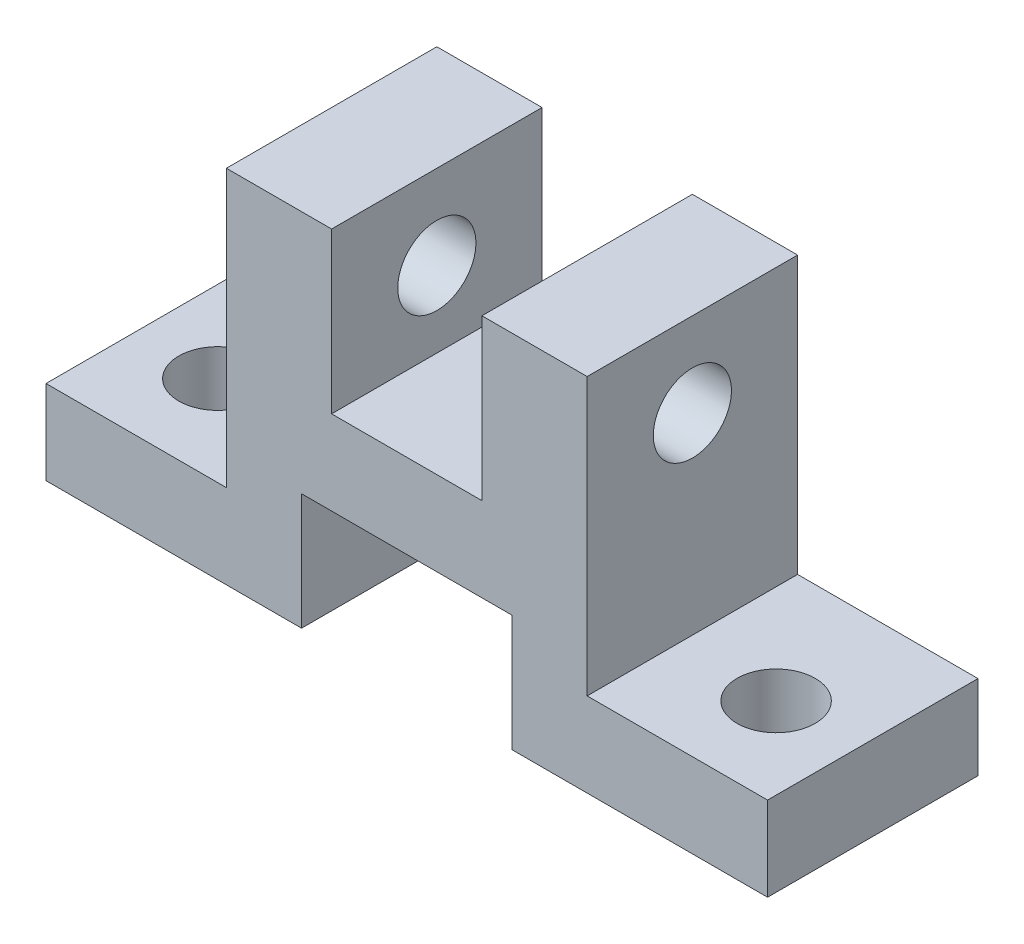
ISO-10303-21;
HEADER;
FILE_DESCRIPTION(('STEP AP214'),'2;1');
FILE_NAME('part.step','',(''),(''),'','','');
FILE_SCHEMA(('AUTOMOTIVE_DESIGN { 1 0 10303 214 1 1 1 1 }'));
ENDSEC;
DATA;
#1=APPLICATION_CONTEXT('core data for automotive mechanical design processes');
#2=APPLICATION_PROTOCOL_DEFINITION('international standard','automotive_design',2000,#1);
#3=PRODUCT_CONTEXT('',#1,'mechanical');
#4=PRODUCT('Part','Part','',(#3));
#5=PRODUCT_RELATED_PRODUCT_CATEGORY('part','',(#4));
#6=PRODUCT_DEFINITION_FORMATION('','',#4);
#7=PRODUCT_DEFINITION_CONTEXT('part definition',#1,'design');
#8=PRODUCT_DEFINITION('design','',#6,#7);
#9=PRODUCT_DEFINITION_SHAPE('','',#8);
#10=(LENGTH_UNIT() NAMED_UNIT(*) SI_UNIT(.MILLI.,.METRE.));
#11=(NAMED_UNIT(*) PLANE_ANGLE_UNIT() SI_UNIT($,.RADIAN.));
#12=(NAMED_UNIT(*) SI_UNIT($,.STERADIAN.) SOLID_ANGLE_UNIT());
#13=UNCERTAINTY_MEASURE_WITH_UNIT(LENGTH_MEASURE(1.E-05),#10,'distance_accuracy_value','');
#14=(GEOMETRIC_REPRESENTATION_CONTEXT(3) GLOBAL_UNCERTAINTY_ASSIGNED_CONTEXT((#13)) GLOBAL_UNIT_ASSIGNED_CONTEXT((#10,
#11,#12)) REPRESENTATION_CONTEXT('',''));
#15=CARTESIAN_POINT('',(0.,0.,0.));
#16=DIRECTION('',(0.,0.,1.));
#17=DIRECTION('',(1.,0.,0.));
#18=AXIS2_PLACEMENT_3D('',#15,#16,#17);
#19=CARTESIAN_POINT('',(0.,0.,35.));
#20=DIRECTION('',(0.,1.,0.));
#21=DIRECTION('',(0.,0.,1.));
#22=AXIS2_PLACEMENT_3D('',#19,#20,#21);
#23=PLANE('',#22);
#24=DIRECTION('',(1.,0.,0.));
#25=VECTOR('',#24,1.);
#26=CARTESIAN_POINT('',(0.,0.,0.));
#27=LINE('',#26,#25);
#28=CARTESIAN_POINT('',(-17.5,0.,0.));
#29=VERTEX_POINT('',#28);
#30=CARTESIAN_POINT('',(17.5,0.,0.));
#31=VERTEX_POINT('',#30);
#32=EDGE_CURVE('E120',#29,#31,#27,.T.);
#33=ORIENTED_EDGE('',*,*,#32,.T.);
#34=DIRECTION('',(0.,0.,-1.));
#35=VECTOR('',#34,1.);
#36=CARTESIAN_POINT('',(17.5,0.,35.));
#37=LINE('',#36,#35);
#38=CARTESIAN_POINT('',(17.5,0.,35.));
#39=VERTEX_POINT('',#38);
#40=EDGE_CURVE('E11',#39,#31,#37,.T.);
#41=ORIENTED_EDGE('',*,*,#40,.F.);
#42=DIRECTION('',(1.,0.,0.));
#43=VECTOR('',#42,1.);
#44=CARTESIAN_POINT('',(0.,0.,35.));
#45=LINE('',#44,#43);
#46=CARTESIAN_POINT('',(-17.5,0.,35.));
#47=VERTEX_POINT('',#46);
#48=EDGE_CURVE('E124',#47,#39,#45,.T.);
#49=ORIENTED_EDGE('',*,*,#48,.F.);
#50=DIRECTION('',(0.,0.,-1.));
#51=VECTOR('',#50,1.);
#52=CARTESIAN_POINT('',(-17.5,0.,35.));
#53=LINE('',#52,#51);
#54=EDGE_CURVE('E182',#47,#29,#53,.T.);
#55=ORIENTED_EDGE('',*,*,#54,.T.);
#56=EDGE_LOOP('',(#33,#41,#49,#55));
#57=FACE_BOUND('',#56,.T.);
#58=ADVANCED_FACE('F41',(#57),#23,.F.);
#59=CARTESIAN_POINT('',(17.5,0.,35.));
#60=DIRECTION('',(1.,0.,0.));
#61=DIRECTION('',(0.,1.,0.));
#62=AXIS2_PLACEMENT_3D('',#59,#60,#61);
#63=PLANE('',#62);
#64=DIRECTION('',(0.,-1.,0.));
#65=VECTOR('',#64,1.);
#66=CARTESIAN_POINT('',(17.5,0.,0.));
#67=LINE('',#66,#65);
#68=CARTESIAN_POINT('',(17.5,-19.3746378464225,0.));
#69=VERTEX_POINT('',#68);
#70=EDGE_CURVE('E188',#31,#69,#67,.T.);
#71=ORIENTED_EDGE('',*,*,#70,.T.);
#72=DIRECTION('',(0.,0.,-1.));
#73=VECTOR('',#72,1.);
#74=CARTESIAN_POINT('',(17.5,-19.3746378464225,35.));
#75=LINE('',#74,#73);
#76=CARTESIAN_POINT('',(17.5,-19.3746378464225,35.));
#77=VERTEX_POINT('',#76);
#78=EDGE_CURVE('E47',#77,#69,#75,.T.);
#79=ORIENTED_EDGE('',*,*,#78,.F.);
#80=DIRECTION('',(0.,-1.,0.));
#81=VECTOR('',#80,1.);
#82=CARTESIAN_POINT('',(17.5,0.,35.));
#83=LINE('',#82,#81);
#84=EDGE_CURVE('E304',#39,#77,#83,.T.);
#85=ORIENTED_EDGE('',*,*,#84,.F.);
#86=ORIENTED_EDGE('',*,*,#40,.T.);
#87=EDGE_LOOP('',(#71,#79,#85,#86));
#88=FACE_BOUND('',#87,.T.);
#89=ADVANCED_FACE('F306',(#88),#63,.F.);
#90=CARTESIAN_POINT('',(17.5,-19.3746378464225,35.));
#91=DIRECTION('',(0.,1.,0.));
#92=DIRECTION('',(-1.,0.,0.));
#93=AXIS2_PLACEMENT_3D('',#90,#91,#92);
#94=PLANE('',#93);
#95=CARTESIAN_POINT('',(46.4238989326504,-19.3746378464225,20.));
#96=DIRECTION('',(0.,1.,0.));
#97=DIRECTION('',(-1.,0.,0.));
#98=AXIS2_PLACEMENT_3D('',#95,#96,#97);
#99=CIRCLE('',#98,6.5);
#100=CARTESIAN_POINT('',(39.9238989326504,-19.3746378464225,20.));
#101=VERTEX_POINT('',#100);
#102=EDGE_CURVE('E379',#101,#101,#99,.T.);
#103=ORIENTED_EDGE('',*,*,#102,.T.);
#104=EDGE_LOOP('',(#103));
#105=FACE_BOUND('',#104,.T.);
#106=DIRECTION('',(1.,0.,0.));
#107=VECTOR('',#106,1.);
#108=CARTESIAN_POINT('',(17.5,-19.3746378464225,0.));
#109=LINE('',#108,#107);
#110=CARTESIAN_POINT('',(60.,-19.3746378464225,0.));
#111=VERTEX_POINT('',#110);
#112=EDGE_CURVE('E189',#69,#111,#109,.T.);
#113=ORIENTED_EDGE('',*,*,#112,.T.);
#114=DIRECTION('',(0.,0.,-1.));
#115=VECTOR('',#114,1.);
#116=CARTESIAN_POINT('',(60.,-19.3746378464225,35.));
#117=LINE('',#116,#115);
#118=CARTESIAN_POINT('',(60.,-19.3746378464225,35.));
#119=VERTEX_POINT('',#118);
#120=EDGE_CURVE('E247',#119,#111,#117,.T.);
#121=ORIENTED_EDGE('',*,*,#120,.F.);
#122=DIRECTION('',(1.,0.,0.));
#123=VECTOR('',#122,1.);
#124=CARTESIAN_POINT('',(17.5,-19.3746378464225,35.));
#125=LINE('',#124,#123);
#126=EDGE_CURVE('E254',#77,#119,#125,.T.);
#127=ORIENTED_EDGE('',*,*,#126,.F.);
#128=ORIENTED_EDGE('',*,*,#78,.T.);
#129=EDGE_LOOP('',(#113,#121,#127,#128));
#130=FACE_BOUND('',#129,.T.);
#131=ADVANCED_FACE('F251',(#105,#130),#94,.F.);
#132=CARTESIAN_POINT('',(60.,-19.3746378464225,35.));
#133=DIRECTION('',(-1.,0.,0.));
#134=DIRECTION('',(0.,0.,1.));
#135=AXIS2_PLACEMENT_3D('',#132,#133,#134);
#136=PLANE('',#135);
#137=DIRECTION('',(0.,1.,0.));
#138=VECTOR('',#137,1.);
#139=CARTESIAN_POINT('',(60.,-19.3746378464225,0.));
#140=LINE('',#139,#138);
#141=CARTESIAN_POINT('',(60.,-5.37463784642245,0.));
#142=VERTEX_POINT('',#141);
#143=EDGE_CURVE('E192',#111,#142,#140,.T.);
#144=ORIENTED_EDGE('',*,*,#143,.T.);
#145=DIRECTION('',(0.,0.,-1.));
#146=VECTOR('',#145,1.);
#147=CARTESIAN_POINT('',(60.,-5.37463784642245,35.));
#148=LINE('',#147,#146);
#149=CARTESIAN_POINT('',(60.,-5.37463784642245,35.));
#150=VERTEX_POINT('',#149);
#151=EDGE_CURVE('E241',#150,#142,#148,.T.);
#152=ORIENTED_EDGE('',*,*,#151,.F.);
#153=DIRECTION('',(0.,1.,0.));
#154=VECTOR('',#153,1.);
#155=CARTESIAN_POINT('',(60.,-19.3746378464225,35.));
#156=LINE('',#155,#154);
#157=EDGE_CURVE('E272',#119,#150,#156,.T.);
#158=ORIENTED_EDGE('',*,*,#157,.F.);
#159=ORIENTED_EDGE('',*,*,#120,.T.);
#160=EDGE_LOOP('',(#144,#152,#158,#159));
#161=FACE_BOUND('',#160,.T.);
#162=ADVANCED_FACE('F262',(#161),#136,.F.);
#163=CARTESIAN_POINT('',(60.,-5.37463784642245,35.));
#164=DIRECTION('',(0.,-1.,0.));
#165=DIRECTION('',(1.,0.,0.));
#166=AXIS2_PLACEMENT_3D('',#163,#164,#165);
#167=PLANE('',#166);
#168=CARTESIAN_POINT('',(46.4238989326504,-5.37463784642245,20.));
#169=DIRECTION('',(0.,1.,0.));
#170=DIRECTION('',(-1.,0.,0.));
#171=AXIS2_PLACEMENT_3D('',#168,#169,#170);
#172=CIRCLE('',#171,6.5);
#173=CARTESIAN_POINT('',(39.9238989326504,-5.37463784642246,20.));
#174=VERTEX_POINT('',#173);
#175=EDGE_CURVE('E382',#174,#174,#172,.T.);
#176=ORIENTED_EDGE('',*,*,#175,.F.);
#177=EDGE_LOOP('',(#176));
#178=FACE_BOUND('',#177,.T.);
#179=DIRECTION('',(-1.,0.,0.));
#180=VECTOR('',#179,1.);
#181=CARTESIAN_POINT('',(60.,-5.37463784642245,0.));
#182=LINE('',#181,#180);
#183=CARTESIAN_POINT('',(30.,-5.37463784642246,0.));
#184=VERTEX_POINT('',#183);
#185=EDGE_CURVE('E194',#142,#184,#182,.T.);
#186=ORIENTED_EDGE('',*,*,#185,.T.);
#187=DIRECTION('',(0.,0.,-1.));
#188=VECTOR('',#187,1.);
#189=CARTESIAN_POINT('',(30.,-5.37463784642246,35.));
#190=LINE('',#189,#188);
#191=CARTESIAN_POINT('',(30.,-5.37463784642246,35.));
#192=VERTEX_POINT('',#191);
#193=EDGE_CURVE('E238',#192,#184,#190,.T.);
#194=ORIENTED_EDGE('',*,*,#193,.F.);
#195=DIRECTION('',(-1.,0.,0.));
#196=VECTOR('',#195,1.);
#197=CARTESIAN_POINT('',(60.,-5.37463784642245,35.));
#198=LINE('',#197,#196);
#199=EDGE_CURVE('E269',#150,#192,#198,.T.);
#200=ORIENTED_EDGE('',*,*,#199,.F.);
#201=ORIENTED_EDGE('',*,*,#151,.T.);
#202=EDGE_LOOP('',(#186,#194,#200,#201));
#203=FACE_BOUND('',#202,.T.);
#204=ADVANCED_FACE('F268',(#178,#203),#167,.F.);
#205=CARTESIAN_POINT('',(30.,-5.37463784642246,35.));
#206=DIRECTION('',(-1.,0.,0.));
#207=DIRECTION('',(0.,0.,1.));
#208=AXIS2_PLACEMENT_3D('',#205,#206,#207);
#209=PLANE('',#208);
#210=CARTESIAN_POINT('',(30.,26.6253621535775,17.5));
#211=DIRECTION('',(-1.,0.,0.));
#212=DIRECTION('',(0.,0.,1.));
#213=AXIS2_PLACEMENT_3D('',#210,#211,#212);
#214=CIRCLE('',#213,6.5);
#215=CARTESIAN_POINT('',(30.,26.6253621535775,24.));
#216=VERTEX_POINT('',#215);
#217=EDGE_CURVE('E190',#216,#216,#214,.T.);
#218=ORIENTED_EDGE('',*,*,#217,.T.);
#219=EDGE_LOOP('',(#218));
#220=FACE_BOUND('',#219,.T.);
#221=DIRECTION('',(0.,1.,0.));
#222=VECTOR('',#221,1.);
#223=CARTESIAN_POINT('',(30.,-5.37463784642246,0.));
#224=LINE('',#223,#222);
#225=CARTESIAN_POINT('',(30.,40.6253621535775,0.));
#226=VERTEX_POINT('',#225);
#227=EDGE_CURVE('E193',#184,#226,#224,.T.);
#228=ORIENTED_EDGE('',*,*,#227,.T.);
#229=DIRECTION('',(0.,0.,-1.));
#230=VECTOR('',#229,1.);
#231=CARTESIAN_POINT('',(30.,40.6253621535775,35.));
#232=LINE('',#231,#230);
#233=CARTESIAN_POINT('',(30.,40.6253621535775,35.));
#234=VERTEX_POINT('',#233);
#235=EDGE_CURVE('E240',#234,#226,#232,.T.);
#236=ORIENTED_EDGE('',*,*,#235,.F.);
#237=DIRECTION('',(0.,1.,0.));
#238=VECTOR('',#237,1.);
#239=CARTESIAN_POINT('',(30.,-5.37463784642246,35.));
#240=LINE('',#239,#238);
#241=EDGE_CURVE('E275',#192,#234,#240,.T.);
#242=ORIENTED_EDGE('',*,*,#241,.F.);
#243=ORIENTED_EDGE('',*,*,#193,.T.);
#244=EDGE_LOOP('',(#228,#236,#242,#243));
#245=FACE_BOUND('',#244,.T.);
#246=ADVANCED_FACE('F321',(#220,#245),#209,.F.);
#247=CARTESIAN_POINT('',(30.,40.6253621535775,35.));
#248=DIRECTION('',(0.,-1.,0.));
#249=DIRECTION('',(0.,0.,-1.));
#250=AXIS2_PLACEMENT_3D('',#247,#248,#249);
#251=PLANE('',#250);
#252=DIRECTION('',(-1.,0.,0.));
#253=VECTOR('',#252,1.);
#254=CARTESIAN_POINT('',(30.,40.6253621535775,0.));
#255=LINE('',#254,#253);
#256=CARTESIAN_POINT('',(12.5,40.6253621535775,0.));
#257=VERTEX_POINT('',#256);
#258=EDGE_CURVE('E197',#226,#257,#255,.T.);
#259=ORIENTED_EDGE('',*,*,#258,.T.);
#260=DIRECTION('',(0.,0.,-1.));
#261=VECTOR('',#260,1.);
#262=CARTESIAN_POINT('',(12.5,40.6253621535775,35.));
#263=LINE('',#262,#261);
#264=CARTESIAN_POINT('',(12.5,40.6253621535775,35.));
#265=VERTEX_POINT('',#264);
#266=EDGE_CURVE('E231',#265,#257,#263,.T.);
#267=ORIENTED_EDGE('',*,*,#266,.F.);
#268=DIRECTION('',(-1.,0.,0.));
#269=VECTOR('',#268,1.);
#270=CARTESIAN_POINT('',(30.,40.6253621535775,35.));
#271=LINE('',#270,#269);
#272=EDGE_CURVE('E274',#234,#265,#271,.T.);
#273=ORIENTED_EDGE('',*,*,#272,.F.);
#274=ORIENTED_EDGE('',*,*,#235,.T.);
#275=EDGE_LOOP('',(#259,#267,#273,#274));
#276=FACE_BOUND('',#275,.T.);
#277=ADVANCED_FACE('F324',(#276),#251,.F.);
#278=CARTESIAN_POINT('',(12.5,40.6253621535775,35.));
#279=DIRECTION('',(1.,0.,0.));
#280=DIRECTION('',(0.,1.,0.));
#281=AXIS2_PLACEMENT_3D('',#278,#279,#280);
#282=PLANE('',#281);
#283=CARTESIAN_POINT('',(12.5,26.6253621535775,17.5));
#284=DIRECTION('',(1.,0.,0.));
#285=DIRECTION('',(0.,1.,0.));
#286=AXIS2_PLACEMENT_3D('',#283,#284,#285);
#287=CIRCLE('',#286,6.5);
#288=CARTESIAN_POINT('',(12.5,26.6253621535775,24.));
#289=VERTEX_POINT('',#288);
#290=EDGE_CURVE('E399',#289,#289,#287,.T.);
#291=ORIENTED_EDGE('',*,*,#290,.T.);
#292=EDGE_LOOP('',(#291));
#293=FACE_BOUND('',#292,.T.);
#294=DIRECTION('',(0.,-1.,0.));
#295=VECTOR('',#294,1.);
#296=CARTESIAN_POINT('',(12.5,40.6253621535775,0.));
#297=LINE('',#296,#295);
#298=CARTESIAN_POINT('',(12.5,14.,0.));
#299=VERTEX_POINT('',#298);
#300=EDGE_CURVE('E200',#257,#299,#297,.T.);
#301=ORIENTED_EDGE('',*,*,#300,.T.);
#302=DIRECTION('',(0.,0.,-1.));
#303=VECTOR('',#302,1.);
#304=CARTESIAN_POINT('',(12.5,14.,35.));
#305=LINE('',#304,#303);
#306=CARTESIAN_POINT('',(12.5,14.,35.));
#307=VERTEX_POINT('',#306);
#308=EDGE_CURVE('E232',#307,#299,#305,.T.);
#309=ORIENTED_EDGE('',*,*,#308,.F.);
#310=DIRECTION('',(0.,-1.,0.));
#311=VECTOR('',#310,1.);
#312=CARTESIAN_POINT('',(12.5,40.6253621535775,35.));
#313=LINE('',#312,#311);
#314=EDGE_CURVE('E283',#265,#307,#313,.T.);
#315=ORIENTED_EDGE('',*,*,#314,.F.);
#316=ORIENTED_EDGE('',*,*,#266,.T.);
#317=EDGE_LOOP('',(#301,#309,#315,#316));
#318=FACE_BOUND('',#317,.T.);
#319=ADVANCED_FACE('F328',(#293,#318),#282,.F.);
#320=CARTESIAN_POINT('',(12.5,14.,35.));
#321=DIRECTION('',(0.,-1.,0.));
#322=DIRECTION('',(0.,0.,-1.));
#323=AXIS2_PLACEMENT_3D('',#320,#321,#322);
#324=PLANE('',#323);
#325=DIRECTION('',(-1.,0.,0.));
#326=VECTOR('',#325,1.);
#327=CARTESIAN_POINT('',(12.5,14.,0.));
#328=LINE('',#327,#326);
#329=CARTESIAN_POINT('',(-12.5,14.,0.));
#330=VERTEX_POINT('',#329);
#331=EDGE_CURVE('E203',#299,#330,#328,.T.);
#332=ORIENTED_EDGE('',*,*,#331,.T.);
#333=DIRECTION('',(0.,0.,-1.));
#334=VECTOR('',#333,1.);
#335=CARTESIAN_POINT('',(-12.5,14.,35.));
#336=LINE('',#335,#334);
#337=CARTESIAN_POINT('',(-12.5,14.,35.));
#338=VERTEX_POINT('',#337);
#339=EDGE_CURVE('E226',#338,#330,#336,.T.);
#340=ORIENTED_EDGE('',*,*,#339,.F.);
#341=DIRECTION('',(-1.,0.,0.));
#342=VECTOR('',#341,1.);
#343=CARTESIAN_POINT('',(12.5,14.,35.));
#344=LINE('',#343,#342);
#345=EDGE_CURVE('E281',#307,#338,#344,.T.);
#346=ORIENTED_EDGE('',*,*,#345,.F.);
#347=ORIENTED_EDGE('',*,*,#308,.T.);
#348=EDGE_LOOP('',(#332,#340,#346,#347));
#349=FACE_BOUND('',#348,.T.);
#350=ADVANCED_FACE('F334',(#349),#324,.F.);
#351=CARTESIAN_POINT('',(-12.5,40.6253621535775,35.));
#352=DIRECTION('',(-1.,0.,0.));
#353=DIRECTION('',(0.,-1.,0.));
#354=AXIS2_PLACEMENT_3D('',#351,#352,#353);
#355=PLANE('',#354);
#356=CARTESIAN_POINT('',(-12.5,26.6253621535775,17.5));
#357=DIRECTION('',(-1.,0.,0.));
#358=DIRECTION('',(0.,-1.,0.));
#359=AXIS2_PLACEMENT_3D('',#356,#357,#358);
#360=CIRCLE('',#359,6.5);
#361=CARTESIAN_POINT('',(-12.5,26.6253621535775,24.));
#362=VERTEX_POINT('',#361);
#363=EDGE_CURVE('E397',#362,#362,#360,.T.);
#364=ORIENTED_EDGE('',*,*,#363,.T.);
#365=EDGE_LOOP('',(#364));
#366=FACE_BOUND('',#365,.T.);
#367=DIRECTION('',(0.,1.,0.));
#368=VECTOR('',#367,1.);
#369=CARTESIAN_POINT('',(-12.5,40.6253621535775,0.));
#370=LINE('',#369,#368);
#371=CARTESIAN_POINT('',(-12.5,40.6253621535775,0.));
#372=VERTEX_POINT('',#371);
#373=EDGE_CURVE('E201',#330,#372,#370,.T.);
#374=ORIENTED_EDGE('',*,*,#373,.T.);
#375=DIRECTION('',(0.,0.,-1.));
#376=VECTOR('',#375,1.);
#377=CARTESIAN_POINT('',(-12.5,40.6253621535775,35.));
#378=LINE('',#377,#376);
#379=CARTESIAN_POINT('',(-12.5,40.6253621535775,35.));
#380=VERTEX_POINT('',#379);
#381=EDGE_CURVE('E223',#380,#372,#378,.T.);
#382=ORIENTED_EDGE('',*,*,#381,.F.);
#383=DIRECTION('',(0.,1.,0.));
#384=VECTOR('',#383,1.);
#385=CARTESIAN_POINT('',(-12.5,40.6253621535775,35.));
#386=LINE('',#385,#384);
#387=EDGE_CURVE('E282',#338,#380,#386,.T.);
#388=ORIENTED_EDGE('',*,*,#387,.F.);
#389=ORIENTED_EDGE('',*,*,#339,.T.);
#390=EDGE_LOOP('',(#374,#382,#388,#389));
#391=FACE_BOUND('',#390,.T.);
#392=ADVANCED_FACE('F340',(#366,#391),#355,.F.);
#393=CARTESIAN_POINT('',(-30.,40.6253621535775,35.));
#394=DIRECTION('',(0.,-1.,0.));
#395=DIRECTION('',(0.,0.,-1.));
#396=AXIS2_PLACEMENT_3D('',#393,#394,#395);
#397=PLANE('',#396);
#398=DIRECTION('',(-1.,0.,0.));
#399=VECTOR('',#398,1.);
#400=CARTESIAN_POINT('',(-30.,40.6253621535775,0.));
#401=LINE('',#400,#399);
#402=CARTESIAN_POINT('',(-30.,40.6253621535775,0.));
#403=VERTEX_POINT('',#402);
#404=EDGE_CURVE('E202',#372,#403,#401,.T.);
#405=ORIENTED_EDGE('',*,*,#404,.T.);
#406=DIRECTION('',(0.,0.,-1.));
#407=VECTOR('',#406,1.);
#408=CARTESIAN_POINT('',(-30.,40.6253621535775,35.));
#409=LINE('',#408,#407);
#410=CARTESIAN_POINT('',(-30.,40.6253621535775,35.));
#411=VERTEX_POINT('',#410);
#412=EDGE_CURVE('E225',#411,#403,#409,.T.);
#413=ORIENTED_EDGE('',*,*,#412,.F.);
#414=DIRECTION('',(-1.,0.,0.));
#415=VECTOR('',#414,1.);
#416=CARTESIAN_POINT('',(-30.,40.6253621535775,35.));
#417=LINE('',#416,#415);
#418=EDGE_CURVE('E290',#380,#411,#417,.T.);
#419=ORIENTED_EDGE('',*,*,#418,.F.);
#420=ORIENTED_EDGE('',*,*,#381,.T.);
#421=EDGE_LOOP('',(#405,#413,#419,#420));
#422=FACE_BOUND('',#421,.T.);
#423=ADVANCED_FACE('F342',(#422),#397,.F.);
#424=CARTESIAN_POINT('',(-30.,-5.37463784642246,35.));
#425=DIRECTION('',(1.,0.,0.));
#426=DIRECTION('',(0.,0.,-1.));
#427=AXIS2_PLACEMENT_3D('',#424,#425,#426);
#428=PLANE('',#427);
#429=CARTESIAN_POINT('',(-30.,26.6253621535775,17.5));
#430=DIRECTION('',(-1.,0.,0.));
#431=DIRECTION('',(0.,0.,1.));
#432=AXIS2_PLACEMENT_3D('',#429,#430,#431);
#433=CIRCLE('',#432,6.5);
#434=CARTESIAN_POINT('',(-30.,26.6253621535775,24.));
#435=VERTEX_POINT('',#434);
#436=EDGE_CURVE('E387',#435,#435,#433,.T.);
#437=ORIENTED_EDGE('',*,*,#436,.F.);
#438=EDGE_LOOP('',(#437));
#439=FACE_BOUND('',#438,.T.);
#440=DIRECTION('',(0.,-1.,0.));
#441=VECTOR('',#440,1.);
#442=CARTESIAN_POINT('',(-30.,-5.37463784642246,0.));
#443=LINE('',#442,#441);
#444=CARTESIAN_POINT('',(-30.,-5.37463784642246,0.));
#445=VERTEX_POINT('',#444);
#446=EDGE_CURVE('E210',#403,#445,#443,.T.);
#447=ORIENTED_EDGE('',*,*,#446,.T.);
#448=DIRECTION('',(0.,0.,-1.));
#449=VECTOR('',#448,1.);
#450=CARTESIAN_POINT('',(-30.,-5.37463784642246,35.));
#451=LINE('',#450,#449);
#452=CARTESIAN_POINT('',(-30.,-5.37463784642246,35.));
#453=VERTEX_POINT('',#452);
#454=EDGE_CURVE('E218',#453,#445,#451,.T.);
#455=ORIENTED_EDGE('',*,*,#454,.F.);
#456=DIRECTION('',(0.,-1.,0.));
#457=VECTOR('',#456,1.);
#458=CARTESIAN_POINT('',(-30.,-5.37463784642246,35.));
#459=LINE('',#458,#457);
#460=EDGE_CURVE('E286',#411,#453,#459,.T.);
#461=ORIENTED_EDGE('',*,*,#460,.F.);
#462=ORIENTED_EDGE('',*,*,#412,.T.);
#463=EDGE_LOOP('',(#447,#455,#461,#462));
#464=FACE_BOUND('',#463,.T.);
#465=ADVANCED_FACE('F293',(#439,#464),#428,.F.);
#466=CARTESIAN_POINT('',(-60.,-5.37463784642245,35.));
#467=DIRECTION('',(0.,-1.,0.));
#468=DIRECTION('',(1.,0.,0.));
#469=AXIS2_PLACEMENT_3D('',#466,#467,#468);
#470=PLANE('',#469);
#471=CARTESIAN_POINT('',(-46.4238989326504,-5.37463784642247,20.));
#472=DIRECTION('',(0.,1.,0.));
#473=DIRECTION('',(1.,0.,0.));
#474=AXIS2_PLACEMENT_3D('',#471,#472,#473);
#475=CIRCLE('',#474,6.5);
#476=CARTESIAN_POINT('',(-39.9238989326504,-5.37463784642246,20.));
#477=VERTEX_POINT('',#476);
#478=EDGE_CURVE('E383',#477,#477,#475,.T.);
#479=ORIENTED_EDGE('',*,*,#478,.F.);
#480=EDGE_LOOP('',(#479));
#481=FACE_BOUND('',#480,.T.);
#482=DIRECTION('',(-1.,0.,0.));
#483=VECTOR('',#482,1.);
#484=CARTESIAN_POINT('',(-60.,-5.37463784642245,0.));
#485=LINE('',#484,#483);
#486=CARTESIAN_POINT('',(-60.,-5.37463784642245,0.));
#487=VERTEX_POINT('',#486);
#488=EDGE_CURVE('E207',#445,#487,#485,.T.);
#489=ORIENTED_EDGE('',*,*,#488,.T.);
#490=DIRECTION('',(0.,0.,-1.));
#491=VECTOR('',#490,1.);
#492=CARTESIAN_POINT('',(-60.,-5.37463784642245,35.));
#493=LINE('',#492,#491);
#494=CARTESIAN_POINT('',(-60.,-5.37463784642245,35.));
#495=VERTEX_POINT('',#494);
#496=EDGE_CURVE('E177',#495,#487,#493,.T.);
#497=ORIENTED_EDGE('',*,*,#496,.F.);
#498=DIRECTION('',(-1.,0.,0.));
#499=VECTOR('',#498,1.);
#500=CARTESIAN_POINT('',(-60.,-5.37463784642245,35.));
#501=LINE('',#500,#499);
#502=EDGE_CURVE('E170',#453,#495,#501,.T.);
#503=ORIENTED_EDGE('',*,*,#502,.F.);
#504=ORIENTED_EDGE('',*,*,#454,.T.);
#505=EDGE_LOOP('',(#489,#497,#503,#504));
#506=FACE_BOUND('',#505,.T.);
#507=ADVANCED_FACE('F299',(#481,#506),#470,.F.);
#508=CARTESIAN_POINT('',(-60.,-19.3746378464225,35.));
#509=DIRECTION('',(1.,0.,0.));
#510=DIRECTION('',(0.,0.,-1.));
#511=AXIS2_PLACEMENT_3D('',#508,#509,#510);
#512=PLANE('',#511);
#513=DIRECTION('',(0.,-1.,0.));
#514=VECTOR('',#513,1.);
#515=CARTESIAN_POINT('',(-60.,-19.3746378464225,0.));
#516=LINE('',#515,#514);
#517=CARTESIAN_POINT('',(-60.,-19.3746378464225,0.));
#518=VERTEX_POINT('',#517);
#519=EDGE_CURVE('E172',#487,#518,#516,.T.);
#520=ORIENTED_EDGE('',*,*,#519,.T.);
#521=DIRECTION('',(0.,0.,-1.));
#522=VECTOR('',#521,1.);
#523=CARTESIAN_POINT('',(-60.,-19.3746378464225,35.));
#524=LINE('',#523,#522);
#525=CARTESIAN_POINT('',(-60.,-19.3746378464225,35.));
#526=VERTEX_POINT('',#525);
#527=EDGE_CURVE('E175',#526,#518,#524,.T.);
#528=ORIENTED_EDGE('',*,*,#527,.F.);
#529=DIRECTION('',(0.,-1.,0.));
#530=VECTOR('',#529,1.);
#531=CARTESIAN_POINT('',(-60.,-19.3746378464225,35.));
#532=LINE('',#531,#530);
#533=EDGE_CURVE('E161',#495,#526,#532,.T.);
#534=ORIENTED_EDGE('',*,*,#533,.F.);
#535=ORIENTED_EDGE('',*,*,#496,.T.);
#536=EDGE_LOOP('',(#520,#528,#534,#535));
#537=FACE_BOUND('',#536,.T.);
#538=ADVANCED_FACE('F171',(#537),#512,.F.);
#539=CARTESIAN_POINT('',(-17.5,-19.3746378464225,35.));
#540=DIRECTION('',(0.,1.,0.));
#541=DIRECTION('',(-1.,0.,0.));
#542=AXIS2_PLACEMENT_3D('',#539,#540,#541);
#543=PLANE('',#542);
#544=CARTESIAN_POINT('',(-46.4238989326504,-19.3746378464225,20.));
#545=DIRECTION('',(0.,1.,0.));
#546=DIRECTION('',(1.,0.,0.));
#547=AXIS2_PLACEMENT_3D('',#544,#545,#546);
#548=CIRCLE('',#547,6.5);
#549=CARTESIAN_POINT('',(-39.9238989326504,-19.3746378464225,20.));
#550=VERTEX_POINT('',#549);
#551=EDGE_CURVE('E386',#550,#550,#548,.T.);
#552=ORIENTED_EDGE('',*,*,#551,.T.);
#553=EDGE_LOOP('',(#552));
#554=FACE_BOUND('',#553,.T.);
#555=DIRECTION('',(1.,0.,0.));
#556=VECTOR('',#555,1.);
#557=CARTESIAN_POINT('',(-17.5,-19.3746378464225,0.));
#558=LINE('',#557,#556);
#559=CARTESIAN_POINT('',(-17.5,-19.3746378464225,0.));
#560=VERTEX_POINT('',#559);
#561=EDGE_CURVE('E109',#518,#560,#558,.T.);
#562=ORIENTED_EDGE('',*,*,#561,.T.);
#563=DIRECTION('',(0.,0.,-1.));
#564=VECTOR('',#563,1.);
#565=CARTESIAN_POINT('',(-17.5,-19.3746378464225,35.));
#566=LINE('',#565,#564);
#567=CARTESIAN_POINT('',(-17.5,-19.3746378464225,35.));
#568=VERTEX_POINT('',#567);
#569=EDGE_CURVE('E180',#568,#560,#566,.T.);
#570=ORIENTED_EDGE('',*,*,#569,.F.);
#571=DIRECTION('',(1.,0.,0.));
#572=VECTOR('',#571,1.);
#573=CARTESIAN_POINT('',(-17.5,-19.3746378464225,35.));
#574=LINE('',#573,#572);
#575=EDGE_CURVE('E164',#526,#568,#574,.T.);
#576=ORIENTED_EDGE('',*,*,#575,.F.);
#577=ORIENTED_EDGE('',*,*,#527,.T.);
#578=EDGE_LOOP('',(#562,#570,#576,#577));
#579=FACE_BOUND('',#578,.T.);
#580=ADVANCED_FACE('F176',(#554,#579),#543,.F.);
#581=CARTESIAN_POINT('',(-17.5,0.,35.));
#582=DIRECTION('',(-1.,0.,0.));
#583=DIRECTION('',(0.,-1.,0.));
#584=AXIS2_PLACEMENT_3D('',#581,#582,#583);
#585=PLANE('',#584);
#586=DIRECTION('',(0.,1.,0.));
#587=VECTOR('',#586,1.);
#588=CARTESIAN_POINT('',(-17.5,0.,0.));
#589=LINE('',#588,#587);
#590=EDGE_CURVE('E213',#560,#29,#589,.T.);
#591=ORIENTED_EDGE('',*,*,#590,.T.);
#592=ORIENTED_EDGE('',*,*,#54,.F.);
#593=DIRECTION('',(0.,1.,0.));
#594=VECTOR('',#593,1.);
#595=CARTESIAN_POINT('',(-17.5,0.,35.));
#596=LINE('',#595,#594);
#597=EDGE_CURVE('E60',#568,#47,#596,.T.);
#598=ORIENTED_EDGE('',*,*,#597,.F.);
#599=ORIENTED_EDGE('',*,*,#569,.T.);
#600=EDGE_LOOP('',(#591,#592,#598,#599));
#601=FACE_BOUND('',#600,.T.);
#602=ADVANCED_FACE('F302',(#601),#585,.F.);
#603=CARTESIAN_POINT('',(0.,0.,35.));
#604=DIRECTION('',(0.,0.,1.));
#605=DIRECTION('',(1.,0.,0.));
#606=AXIS2_PLACEMENT_3D('',#603,#604,#605);
#607=PLANE('',#606);
#608=ORIENTED_EDGE('',*,*,#48,.T.);
#609=ORIENTED_EDGE('',*,*,#84,.T.);
#610=ORIENTED_EDGE('',*,*,#126,.T.);
#611=ORIENTED_EDGE('',*,*,#157,.T.);
#612=ORIENTED_EDGE('',*,*,#199,.T.);
#613=ORIENTED_EDGE('',*,*,#241,.T.);
#614=ORIENTED_EDGE('',*,*,#272,.T.);
#615=ORIENTED_EDGE('',*,*,#314,.T.);
#616=ORIENTED_EDGE('',*,*,#345,.T.);
#617=ORIENTED_EDGE('',*,*,#387,.T.);
#618=ORIENTED_EDGE('',*,*,#418,.T.);
#619=ORIENTED_EDGE('',*,*,#460,.T.);
#620=ORIENTED_EDGE('',*,*,#502,.T.);
#621=ORIENTED_EDGE('',*,*,#533,.T.);
#622=ORIENTED_EDGE('',*,*,#575,.T.);
#623=ORIENTED_EDGE('',*,*,#597,.T.);
#624=EDGE_LOOP('',(#608,#609,#610,#611,#612,#613,#614,#615,#616,#617,#618,#619,#620,#621,#622,#623));
#625=FACE_BOUND('',#624,.T.);
#626=ADVANCED_FACE('F162',(#625),#607,.T.);
#627=CARTESIAN_POINT('',(0.,0.,0.));
#628=DIRECTION('',(0.,0.,1.));
#629=DIRECTION('',(1.,0.,0.));
#630=AXIS2_PLACEMENT_3D('',#627,#628,#629);
#631=PLANE('',#630);
#632=ORIENTED_EDGE('',*,*,#32,.F.);
#633=ORIENTED_EDGE('',*,*,#590,.F.);
#634=ORIENTED_EDGE('',*,*,#561,.F.);
#635=ORIENTED_EDGE('',*,*,#519,.F.);
#636=ORIENTED_EDGE('',*,*,#488,.F.);
#637=ORIENTED_EDGE('',*,*,#446,.F.);
#638=ORIENTED_EDGE('',*,*,#404,.F.);
#639=ORIENTED_EDGE('',*,*,#373,.F.);
#640=ORIENTED_EDGE('',*,*,#331,.F.);
#641=ORIENTED_EDGE('',*,*,#300,.F.);
#642=ORIENTED_EDGE('',*,*,#258,.F.);
#643=ORIENTED_EDGE('',*,*,#227,.F.);
#644=ORIENTED_EDGE('',*,*,#185,.F.);
#645=ORIENTED_EDGE('',*,*,#143,.F.);
#646=ORIENTED_EDGE('',*,*,#112,.F.);
#647=ORIENTED_EDGE('',*,*,#70,.F.);
#648=EDGE_LOOP('',(#632,#633,#634,#635,#636,#637,#638,#639,#640,#641,#642,#643,#644,#645,#646,#647));
#649=FACE_BOUND('',#648,.T.);
#650=ADVANCED_FACE('F259',(#649),#631,.F.);
#651=CARTESIAN_POINT('',(60.,26.6253621535775,17.5));
#652=DIRECTION('',(-1.,0.,0.));
#653=DIRECTION('',(0.,0.,1.));
#654=AXIS2_PLACEMENT_3D('',#651,#652,#653);
#655=CYLINDRICAL_SURFACE('',#654,6.5);
#656=CARTESIAN_POINT('',(-30.,26.6253621535775,24.));
#657=CARTESIAN_POINT('',(-29.8177083333333,26.6253621535775,24.));
#658=CARTESIAN_POINT('',(-29.6354166666667,26.6253621535775,24.));
#659=CARTESIAN_POINT('',(-29.2708333333333,26.6253621535775,24.));
#660=CARTESIAN_POINT('',(-29.0885416666666,26.6253621535775,24.));
#661=CARTESIAN_POINT('',(-28.7239583333333,26.6253621535775,24.));
#662=CARTESIAN_POINT('',(-28.5416666666667,26.6253621535775,24.));
#663=CARTESIAN_POINT('',(-28.1770833333333,26.6253621535775,24.));
#664=CARTESIAN_POINT('',(-27.9947916666667,26.6253621535775,24.));
#665=CARTESIAN_POINT('',(-27.6302083333333,26.6253621535775,24.));
#666=CARTESIAN_POINT('',(-27.4479166666667,26.6253621535775,24.));
#667=CARTESIAN_POINT('',(-27.0833333333333,26.6253621535775,24.));
#668=CARTESIAN_POINT('',(-26.9010416666667,26.6253621535775,24.));
#669=CARTESIAN_POINT('',(-26.5364583333333,26.6253621535775,24.));
#670=CARTESIAN_POINT('',(-26.3541666666667,26.6253621535775,24.));
#671=CARTESIAN_POINT('',(-25.9895833333333,26.6253621535775,24.));
#672=CARTESIAN_POINT('',(-25.8072916666667,26.6253621535775,24.));
#673=CARTESIAN_POINT('',(-25.4427083333333,26.6253621535775,24.));
#674=CARTESIAN_POINT('',(-25.2604166666667,26.6253621535775,24.));
#675=CARTESIAN_POINT('',(-24.8958333333333,26.6253621535775,24.));
#676=CARTESIAN_POINT('',(-24.7135416666667,26.6253621535775,24.));
#677=CARTESIAN_POINT('',(-24.3489583333333,26.6253621535775,24.));
#678=CARTESIAN_POINT('',(-24.1666666666667,26.6253621535775,24.));
#679=CARTESIAN_POINT('',(-23.8020833333333,26.6253621535775,24.));
#680=CARTESIAN_POINT('',(-23.6197916666667,26.6253621535775,24.));
#681=CARTESIAN_POINT('',(-23.2552083333333,26.6253621535775,24.));
#682=CARTESIAN_POINT('',(-23.0729166666667,26.6253621535775,24.));
#683=CARTESIAN_POINT('',(-22.7083333333333,26.6253621535775,24.));
#684=CARTESIAN_POINT('',(-22.5260416666667,26.6253621535775,24.));
#685=CARTESIAN_POINT('',(-22.1614583333333,26.6253621535775,24.));
#686=CARTESIAN_POINT('',(-21.9791666666667,26.6253621535775,24.));
#687=CARTESIAN_POINT('',(-21.6145833333333,26.6253621535775,24.));
#688=CARTESIAN_POINT('',(-21.4322916666667,26.6253621535775,24.));
#689=CARTESIAN_POINT('',(-21.0677083333333,26.6253621535775,24.));
#690=CARTESIAN_POINT('',(-20.8854166666667,26.6253621535775,24.));
#691=CARTESIAN_POINT('',(-20.5208333333333,26.6253621535775,24.));
#692=CARTESIAN_POINT('',(-20.3385416666667,26.6253621535775,24.));
#693=CARTESIAN_POINT('',(-19.9739583333333,26.6253621535775,24.));
#694=CARTESIAN_POINT('',(-19.7916666666667,26.6253621535775,24.));
#695=CARTESIAN_POINT('',(-19.4270833333333,26.6253621535775,24.));
#696=CARTESIAN_POINT('',(-19.2447916666667,26.6253621535775,24.));
#697=CARTESIAN_POINT('',(-18.8802083333333,26.6253621535775,24.));
#698=CARTESIAN_POINT('',(-18.6979166666667,26.6253621535775,24.));
#699=CARTESIAN_POINT('',(-18.3333333333333,26.6253621535775,24.));
#700=CARTESIAN_POINT('',(-18.1510416666667,26.6253621535775,24.));
#701=CARTESIAN_POINT('',(-17.7864583333333,26.6253621535775,24.));
#702=CARTESIAN_POINT('',(-17.6041666666667,26.6253621535775,24.));
#703=CARTESIAN_POINT('',(-17.2395833333333,26.6253621535775,24.));
#704=CARTESIAN_POINT('',(-17.0572916666667,26.6253621535775,24.));
#705=CARTESIAN_POINT('',(-16.6927083333333,26.6253621535775,24.));
#706=CARTESIAN_POINT('',(-16.5104166666667,26.6253621535775,24.));
#707=CARTESIAN_POINT('',(-16.1458333333333,26.6253621535775,24.));
#708=CARTESIAN_POINT('',(-15.9635416666667,26.6253621535775,24.));
#709=CARTESIAN_POINT('',(-15.5989583333333,26.6253621535775,24.));
#710=CARTESIAN_POINT('',(-15.4166666666667,26.6253621535775,24.));
#711=CARTESIAN_POINT('',(-15.0520833333333,26.6253621535775,24.));
#712=CARTESIAN_POINT('',(-14.8697916666667,26.6253621535775,24.));
#713=CARTESIAN_POINT('',(-14.5052083333333,26.6253621535775,24.));
#714=CARTESIAN_POINT('',(-14.3229166666667,26.6253621535775,24.));
#715=CARTESIAN_POINT('',(-13.9583333333333,26.6253621535775,24.));
#716=CARTESIAN_POINT('',(-13.7760416666667,26.6253621535775,24.));
#717=CARTESIAN_POINT('',(-13.4114583333333,26.6253621535775,24.));
#718=CARTESIAN_POINT('',(-13.2291666666667,26.6253621535775,24.));
#719=CARTESIAN_POINT('',(-12.8645833333333,26.6253621535775,24.));
#720=CARTESIAN_POINT('',(-12.6822916666667,26.6253621535775,24.));
#721=CARTESIAN_POINT('',(-12.5,26.6253621535775,24.));
#722=B_SPLINE_CURVE_WITH_KNOTS('',3,(#656,#657,#658,#659,#660,#661,#662,#663,#664,#665,#666,
#667,#668,#669,#670,#671,#672,#673,#674,#675,#676,#677,#678,#679,#680,#681,#682,#683,#684,#685,
#686,#687,#688,#689,#690,#691,#692,#693,#694,#695,#696,#697,#698,#699,#700,#701,#702,#703,#704,
#705,#706,#707,#708,#709,#710,#711,#712,#713,#714,#715,#716,#717,#718,#719,#720,#721),
.UNSPECIFIED.,.F.,.F.,(4,2,2,2,2,2,2,2,2,2,2,2,2,2,2,2,2,2,2,2,2,2,2,2,2,2,2,2,2,2,2,2,4),(0.,
0.546875000000002,1.09375,1.64062499999999,2.1875,2.734375,3.28125,3.828125,4.37499999999999,
4.92187499999999,5.46874999999999,6.015625,6.5625,7.109375,7.65624999999999,8.20312499999999,
8.74999999999999,9.296875,9.84375,10.390625,10.9375,11.484375,12.03125,12.578125,13.125,
13.671875,14.21875,14.765625,15.3125,15.859375,16.40625,16.953125,17.5),.UNSPECIFIED.);
#723=EDGE_CURVE('BSEAM363',#435,#362,#722,.T.);
#724=ORIENTED_EDGE('',*,*,#436,.T.);
#725=ORIENTED_EDGE('',*,*,#363,.F.);
#726=ORIENTED_EDGE('',*,*,#723,.T.);
#727=ORIENTED_EDGE('',*,*,#723,.F.);
#728=EDGE_LOOP('',(#724,#726,#725,#727));
#729=FACE_BOUND('',#728,.T.);
#730=ADVANCED_FACE('F363',(#729),#655,.F.);
#731=CARTESIAN_POINT('',(12.5,26.6253621535775,24.));
#732=CARTESIAN_POINT('',(12.6822916666667,26.6253621535775,24.));
#733=CARTESIAN_POINT('',(12.8645833333333,26.6253621535775,24.));
#734=CARTESIAN_POINT('',(13.2291666666667,26.6253621535775,24.));
#735=CARTESIAN_POINT('',(13.4114583333333,26.6253621535775,24.));
#736=CARTESIAN_POINT('',(13.7760416666667,26.6253621535775,24.));
#737=CARTESIAN_POINT('',(13.9583333333333,26.6253621535775,24.));
#738=CARTESIAN_POINT('',(14.3229166666667,26.6253621535775,24.));
#739=CARTESIAN_POINT('',(14.5052083333333,26.6253621535775,24.));
#740=CARTESIAN_POINT('',(14.8697916666667,26.6253621535775,24.));
#741=CARTESIAN_POINT('',(15.0520833333333,26.6253621535775,24.));
#742=CARTESIAN_POINT('',(15.4166666666667,26.6253621535775,24.));
#743=CARTESIAN_POINT('',(15.5989583333333,26.6253621535775,24.));
#744=CARTESIAN_POINT('',(15.9635416666667,26.6253621535775,24.));
#745=CARTESIAN_POINT('',(16.1458333333333,26.6253621535775,24.));
#746=CARTESIAN_POINT('',(16.5104166666667,26.6253621535775,24.));
#747=CARTESIAN_POINT('',(16.6927083333333,26.6253621535775,24.));
#748=CARTESIAN_POINT('',(17.0572916666667,26.6253621535775,24.));
#749=CARTESIAN_POINT('',(17.2395833333333,26.6253621535775,24.));
#750=CARTESIAN_POINT('',(17.6041666666667,26.6253621535775,24.));
#751=CARTESIAN_POINT('',(17.7864583333333,26.6253621535775,24.));
#752=CARTESIAN_POINT('',(18.1510416666667,26.6253621535775,24.));
#753=CARTESIAN_POINT('',(18.3333333333333,26.6253621535775,24.));
#754=CARTESIAN_POINT('',(18.6979166666667,26.6253621535775,24.));
#755=CARTESIAN_POINT('',(18.8802083333333,26.6253621535775,24.));
#756=CARTESIAN_POINT('',(19.2447916666667,26.6253621535775,24.));
#757=CARTESIAN_POINT('',(19.4270833333333,26.6253621535775,24.));
#758=CARTESIAN_POINT('',(19.7916666666667,26.6253621535775,24.));
#759=CARTESIAN_POINT('',(19.9739583333333,26.6253621535775,24.));
#760=CARTESIAN_POINT('',(20.3385416666667,26.6253621535775,24.));
#761=CARTESIAN_POINT('',(20.5208333333333,26.6253621535775,24.));
#762=CARTESIAN_POINT('',(20.8854166666667,26.6253621535775,24.));
#763=CARTESIAN_POINT('',(21.0677083333333,26.6253621535775,24.));
#764=CARTESIAN_POINT('',(21.4322916666667,26.6253621535775,24.));
#765=CARTESIAN_POINT('',(21.6145833333333,26.6253621535775,24.));
#766=CARTESIAN_POINT('',(21.9791666666667,26.6253621535775,24.));
#767=CARTESIAN_POINT('',(22.1614583333333,26.6253621535775,24.));
#768=CARTESIAN_POINT('',(22.5260416666667,26.6253621535775,24.));
#769=CARTESIAN_POINT('',(22.7083333333333,26.6253621535775,24.));
#770=CARTESIAN_POINT('',(23.0729166666667,26.6253621535775,24.));
#771=CARTESIAN_POINT('',(23.2552083333333,26.6253621535775,24.));
#772=CARTESIAN_POINT('',(23.6197916666667,26.6253621535775,24.));
#773=CARTESIAN_POINT('',(23.8020833333333,26.6253621535775,24.));
#774=CARTESIAN_POINT('',(24.1666666666667,26.6253621535775,24.));
#775=CARTESIAN_POINT('',(24.3489583333333,26.6253621535775,24.));
#776=CARTESIAN_POINT('',(24.7135416666667,26.6253621535775,24.));
#777=CARTESIAN_POINT('',(24.8958333333333,26.6253621535775,24.));
#778=CARTESIAN_POINT('',(25.2604166666667,26.6253621535775,24.));
#779=CARTESIAN_POINT('',(25.4427083333333,26.6253621535775,24.));
#780=CARTESIAN_POINT('',(25.8072916666667,26.6253621535775,24.));
#781=CARTESIAN_POINT('',(25.9895833333333,26.6253621535775,24.));
#782=CARTESIAN_POINT('',(26.3541666666667,26.6253621535775,24.));
#783=CARTESIAN_POINT('',(26.5364583333333,26.6253621535775,24.));
#784=CARTESIAN_POINT('',(26.9010416666667,26.6253621535775,24.));
#785=CARTESIAN_POINT('',(27.0833333333333,26.6253621535775,24.));
#786=CARTESIAN_POINT('',(27.4479166666667,26.6253621535775,24.));
#787=CARTESIAN_POINT('',(27.6302083333333,26.6253621535775,24.));
#788=CARTESIAN_POINT('',(27.9947916666667,26.6253621535775,24.));
#789=CARTESIAN_POINT('',(28.1770833333333,26.6253621535775,24.));
#790=CARTESIAN_POINT('',(28.5416666666667,26.6253621535775,24.));
#791=CARTESIAN_POINT('',(28.7239583333333,26.6253621535775,24.));
#792=CARTESIAN_POINT('',(29.0885416666667,26.6253621535775,24.));
#793=CARTESIAN_POINT('',(29.2708333333333,26.6253621535775,24.));
#794=CARTESIAN_POINT('',(29.6354166666667,26.6253621535775,24.));
#795=CARTESIAN_POINT('',(29.8177083333333,26.6253621535775,24.));
#796=CARTESIAN_POINT('',(30.,26.6253621535775,24.));
#797=B_SPLINE_CURVE_WITH_KNOTS('',3,(#731,#732,#733,#734,#735,#736,#737,#738,#739,#740,#741,
#742,#743,#744,#745,#746,#747,#748,#749,#750,#751,#752,#753,#754,#755,#756,#757,#758,#759,#760,
#761,#762,#763,#764,#765,#766,#767,#768,#769,#770,#771,#772,#773,#774,#775,#776,#777,#778,#779,
#780,#781,#782,#783,#784,#785,#786,#787,#788,#789,#790,#791,#792,#793,#794,#795,#796),
.UNSPECIFIED.,.F.,.F.,(4,2,2,2,2,2,2,2,2,2,2,2,2,2,2,2,2,2,2,2,2,2,2,2,2,2,2,2,2,2,2,2,4),(0.,
0.546875000000002,1.09375,1.640625,2.1875,2.734375,3.28125,3.828125,4.375,4.92187500000001,
5.46875000000001,6.015625,6.56250000000001,7.10937500000001,7.65625,8.20312500000001,
8.75000000000001,9.29687500000001,9.84375000000001,10.390625,10.9375,11.484375,12.03125,
12.578125,13.125,13.671875,14.21875,14.765625,15.3125,15.859375,16.40625,16.953125,17.5),.UNSPECIFIED.);
#798=EDGE_CURVE('BSEAM365',#289,#216,#797,.T.);
#799=ORIENTED_EDGE('',*,*,#290,.F.);
#800=ORIENTED_EDGE('',*,*,#217,.F.);
#801=ORIENTED_EDGE('',*,*,#798,.T.);
#802=ORIENTED_EDGE('',*,*,#798,.F.);
#803=EDGE_LOOP('',(#799,#801,#800,#802));
#804=FACE_BOUND('',#803,.T.);
#805=ADVANCED_FACE('F365',(#804),#655,.F.);
#806=CARTESIAN_POINT('',(-46.4238989326504,-19.3746378464225,20.));
#807=DIRECTION('',(0.,1.,0.));
#808=DIRECTION('',(-1.,0.,0.));
#809=AXIS2_PLACEMENT_3D('',#806,#807,#808);
#810=CYLINDRICAL_SURFACE('',#809,6.5);
#811=ORIENTED_EDGE('',*,*,#551,.F.);
#812=EDGE_LOOP('',(#811));
#813=FACE_BOUND('',#812,.T.);
#814=ORIENTED_EDGE('',*,*,#478,.T.);
#815=EDGE_LOOP('',(#814));
#816=FACE_BOUND('',#815,.T.);
#817=ADVANCED_FACE('F370',(#813,#816),#810,.F.);
#818=CARTESIAN_POINT('',(46.4238989326504,-19.3746378464225,20.));
#819=DIRECTION('',(0.,1.,0.));
#820=DIRECTION('',(-1.,0.,0.));
#821=AXIS2_PLACEMENT_3D('',#818,#819,#820);
#822=CYLINDRICAL_SURFACE('',#821,6.5);
#823=ORIENTED_EDGE('',*,*,#102,.F.);
#824=EDGE_LOOP('',(#823));
#825=FACE_BOUND('',#824,.T.);
#826=ORIENTED_EDGE('',*,*,#175,.T.);
#827=EDGE_LOOP('',(#826));
#828=FACE_BOUND('',#827,.T.);
#829=ADVANCED_FACE('F371',(#825,#828),#822,.F.);
#830=CLOSED_SHELL('',(#58,#89,#131,#162,#204,#246,#277,#319,#350,#392,#423,#465,#507,#538,#580,
#602,#626,#650,#730,#805,#817,#829));
#831=MANIFOLD_SOLID_BREP('B2',#830);
#832=ADVANCED_BREP_SHAPE_REPRESENTATION('',(#18,#831),#14);
#833=SHAPE_DEFINITION_REPRESENTATION(#9,#832);
ENDSEC;
END-ISO-10303-21;
